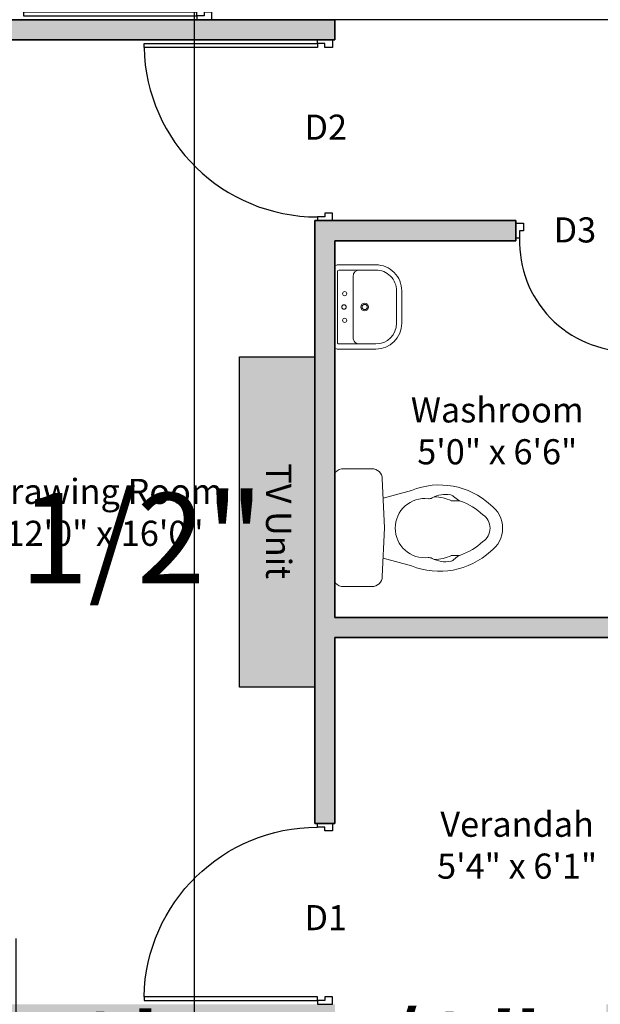
# Model space of a CAD drawing. Units: inches. Extents: x 2796 to 3603, y 978 to 1787.
# Tile 5 of 15: x 3165 to 3280, y 1116 to 1312. Entities that reach past the tile are written whole.
import ezdxf

# ---------------------------------------------------------------- set-up
doc = ezdxf.new("R2010")
doc.units = ezdxf.units.IN
for name, color, linetype, lineweight in [('A-ANNO-DIMS', 7, 'Continuous', 18), ('A-ANNO-TEXT', 7, 'Continuous', 18), ('A-AREA-IDEN', 7, 'Continuous', 18), ('A-DOOR', 6, 'Continuous', 25), ('A-FLOR-CASE', 2, 'Continuous', 25), ('A-FLOR-CASE-PATT', 2, 'Continuous', 13), ('A-FLOR-FIXT', 8, 'Continuous', 18), ('A-WALL-EXTR-PATT', 1, 'Continuous', 13), ('A-WALL-INTR-PATT', 5, 'Continuous', 13), ('Inner Wall', 5, 'Continuous', 35)]:
    doc.layers.add(name, color=color, linetype=linetype, lineweight=lineweight)
doc.styles.get("Standard").update_dxf_attribs({"font": 'arial.ttf'})
doc.dimstyles.get("Standard").update_dxf_attribs({"dimtxt": 18, "dimasz": 12, "dimexe": 0.18, "dimexo": 0.0625, "dimgap": 0.09, "dimtad": 0, "dimtih": 1, "dimtoh": 1, "dimdec": 0, "dimzin": 0, "dimdsep": 46, "dimlunit": 3, "dimtxsty": 'Standard', "dimcen": 0.09, "dimadec": 0, "dimazin": 0, "dimtfac": 1, "dimtdec": 0, "dimtofl": 0, "dimtmove": 0, "dimatfit": 3, "dimfxl": 1, "dimtolj": 1, "dimtzin": 0, "dimarcsym": 0})

# ---------------------------------------------------------------- blocks, each defined once
blk = doc.blocks.new('A$C57EA129C')
for p, q in [((0, 0.4428), (0, 0.1782)), ((0.016, 0.4589), (0.5631, 0.4589)), ((0.0356, 0.4321), (0.0356, 0.2896)), ((0.0445, 0.441), (0.5346, 0.441)), ((0.5435, 0.4321), (0.5435, 0.2896)), ((0.5791, 0.4428), (0.5791, 0.1782)), ((0.0356, 0.2896), (0.0356, 0.1782)), ((0.0802, 0.3341), (0.499, 0.3341)), ((0.5435, 0.2896), (0.5435, 0.1782)), ((0.1782, 0.0356), (0.4009, 0.0356)), ((0.1782, 0), (0.4009, 0))]:
    blk.add_line(p, q)
for centre, radius in [((0.1982, 0.392), 0.0143), ((0.2896, 0.3965), 0.0156), ((0.3809, 0.392), 0.0143), ((0.2896, 0.2545), 0.0267), ((0.2896, 0.2545), 0.0178)]:
    blk.add_circle(centre, radius)
for centre, radius, start, end in [((0.016, 0.4428), 0.016, 90, 180), ((0.0445, 0.4321), 0.00891, 90, 180), ((0.5346, 0.4321), 0.00891, 0, 90), ((0.5631, 0.4428), 0.016, 0, 90), ((0.0802, 0.2896), 0.0445, 90, 180), ((0.499, 0.2896), 0.0445, 0, 90), ((0.1782, 0.1782), 0.1782, 180, 270), ((0.1782, 0.1782), 0.1426, 180, 270), ((0.4009, 0.1782), 0.1782, 270, 0), ((0.4009, 0.1782), 0.1426, 270, 0)]:
    blk.add_arc(centre, radius, start, end)
blk = doc.blocks.new('A$C1308471B')
at = {"ltscale": 20}
for p, q in [((0, 0.4607), (0, 0.0186)), ((0.0354, 0.4793), (0.1495, 0.4793)), ((0.2013, 0.2397), (0.1923, 0.4384)), ((0.1957, 0.3639), (0.3109, 0.3953)), ((0.4982, 0.3575), (0.4822, 0.3709)), ((0.5021, 0.3528), (0.4724, 0.3528)), ((0.2013, 0.2397), (0.1923, 0.0409)), ((0.5021, 0.1304), (0.4724, 0.1304)), ((0.4982, 0.1257), (0.4822, 0.1123)), ((0.1959, 0.1193), (0.3109, 0.0879)), ((0.0354, 0), (0.1495, 0))]:
    blk.add_line(p, q, dxfattribs=at)
for centre, radius, start, end in [((0.006, 0.4607), 0.006, 136.5269, 180), ((0.0354, 0.4328), 0.0465, 90, 136.5269), ((0.1495, 0.4365), 0.0429, 2.5755, 90), ((0.4248, 0.1104), 0.3068, 47.4135, 111.7924), ((0.3654, 0.2416), 0.1206, 83.3523, 180), ((0.3823, 0.3868), 0.0255, 263.3523, 298.5742), ((0.4494, 0.2636), 0.1148, 79.3968, 118.5742), ((0.405, 0.2159), 0.153, 63.502, 90.4522), ((0.4658, 0.3513), 0.0255, 50, 79.3968), ((0.5146, 0.377), 0.0255, 230, 251.3881), ((0.5021, 0.3273), 0.0255, 70.3751, 90), ((0.4248, 0.1104), 0.2558, 46.612, 70.3751), ((0.5654, 0.2416), 0.116, 0, 54.7115), ((0.5654, 0.2416), 0.065, 0, 57.2974), ((0.3654, 0.2416), 0.1206, 180, 276.6477), ((0.5654, 0.2416), 0.065, 302.7026, 0), ((0.5654, 0.2416), 0.116, 305.2885, 0), ((0.4248, 0.3728), 0.2558, 289.6249, 313.388), ((0.4248, 0.3728), 0.3068, 248.2076, 312.5865), ((0.3823, 0.0964), 0.0255, 61.4258, 96.6477), ((0.405, 0.2673), 0.153, 269.5478, 296.498), ((0.5146, 0.1062), 0.0255, 108.6119, 130), ((0.5021, 0.1559), 0.0255, 270, 289.6249), ((0.4494, 0.2196), 0.1148, 241.4258, 280.6032), ((0.4658, 0.1319), 0.0255, 280.6032, 310), ((0.1495, 0.0429), 0.0429, 270, 357.4245), ((0.006, 0.0186), 0.006, 180, 223.4731), ((0.0354, 0.0465), 0.0465, 223.4731, 270)]:
    blk.add_arc(centre, radius, start, end, dxfattribs=at)
blk = doc.blocks.new('DOOR-SWING-36IN')
for points in [[(-0.01, 34.5), (-0.01, 0), (-0.76, 0), (-0.76, 34.5)], [(-35.26, -3), (-33.76, -3), (-33.76, -1.5), (-34.51, -1.5), (-34.51, 0), (-35.26, 0)], [(0.74, -3), (-0.76, -3), (-0.76, -1.5), (-0.01, -1.5), (-0.01, 0), (0.74, 0)]]:
    blk.add_lwpolyline(points, close=True)
blk.add_arc((0, 0), 34.51, 91.2592, 180)
blk = doc.blocks.new('DOOR-SWING-24IN')
for points in [[(-0.75, -0.7375), (-0.75, 21.7625), (0, 21.7625), (0, -0.7375)], [(-1.5, -3.7375), (0, -3.7375), (0, -2.2375), (-0.75, -2.2375), (-0.75, -0.7375), (-1.5, -0.7375)], [(22.5, -3.7375), (21, -3.7375), (21, -2.2375), (21.75, -2.2375), (21.75, -0.7375), (22.5, -0.7375)]]:
    blk.add_lwpolyline(points, close=True)
blk.add_arc((0, 0), 21.7625, 358.057956, 90)
blk = doc.blocks.new('TV-UNIT-66IN-NOM')
blk.add_lwpolyline([(0, 0), (65.77, 0), (65.77, -15), (0, -15)], close=True)
blk = doc.blocks.new('*D30')
at = {"layer": 'A-ANNO-DIMS', "color": 0, "lineweight": -2, "transparency": 16777216}
for p, q in [((3083.98, 1288.1), (3059.97, 1288.1)), ((3060.15, 1276.1), (3060.15, 1217.86)), ((3060.15, 1140.81), (3060.15, 1199.05)), ((3083.98, 1128.81), (3059.97, 1128.81))]:
    blk.add_line(p, q, dxfattribs=at)
at = {"layer": 'A-ANNO-DIMS', "color": 0, "transparency": 16777216}
for points in [[(3058.15, 1276.1), (3062.15, 1276.1), (3060.15, 1288.1)], [(3058.15, 1140.81), (3062.15, 1140.81), (3060.15, 1128.81)]]:
    blk.add_solid(points, dxfattribs=at)
at = {"layer": 'Defpoints', "color": 0, "transparency": 16777216}
for p in [(3084.05, 1288.1), (3060.15, 1128.81), (3084.05, 1128.81)]:
    blk.add_point(p, dxfattribs=at)
at = {"layer": 'A-ANNO-DIMS', "color": 0, "transparency": 16777216, "insert": (3060.15, 1208.46), "char_height": 18, "attachment_point": 5}
blk.add_mtext('\\A1;SEATING GROUP 13\'-3 1/2"', dxfattribs=at)
blk = doc.blocks.new('*D31')
at = {"layer": 'A-ANNO-DIMS', "color": 0, "lineweight": -2, "transparency": 16777216}
for p, q in [((3084.05, 1128.75), (3084.05, 1104.74)), ((3163.77, 1128.75), (3163.77, 1104.74)), ((3096.05, 1104.92), (3151.77, 1104.92)), ((3163.77, 1104.92), (3175.77, 1104.92))]:
    blk.add_line(p, q, dxfattribs=at)
at = {"layer": 'A-ANNO-DIMS', "color": 0, "transparency": 16777216}
for points in [[(3096.05, 1106.92), (3096.05, 1102.92), (3084.05, 1104.92)], [(3151.77, 1106.92), (3151.77, 1102.92), (3163.77, 1104.92)]]:
    blk.add_solid(points, dxfattribs=at)
at = {"layer": 'Defpoints', "color": 0, "transparency": 16777216}
for p in [(3084.05, 1128.81), (3163.77, 1128.81), (3163.77, 1104.92)]:
    blk.add_point(p, dxfattribs=at)
at = {"layer": 'A-ANNO-DIMS', "color": 0, "transparency": 16777216, "insert": (3220.81, 1104.92), "char_height": 18, "attachment_point": 5}
blk.add_mtext('\\A1;6\'-7 1/2"', dxfattribs=at)
blk = doc.blocks.new('*D34')
at = {"layer": 'A-ANNO-DIMS', "color": 0, "lineweight": -2, "transparency": 16777216}
for p, q in [((3355.83, 1336.87), (3343.83, 1336.87)), ((3355.83, 1332.81), (3355.83, 1337.05)), ((3371.32, 1336.87), (3367.83, 1336.87)), ((3383.32, 1332.81), (3383.32, 1337.05))]:
    blk.add_line(p, q, dxfattribs=at)
at = {"layer": 'A-ANNO-DIMS', "color": 0, "transparency": 16777216}
for points in [[(3367.83, 1338.87), (3367.83, 1334.87), (3355.83, 1336.87)], [(3371.32, 1338.87), (3371.32, 1334.87), (3383.32, 1336.87)]]:
    blk.add_solid(points, dxfattribs=at)
at = {"layer": 'Defpoints', "color": 0, "transparency": 16777216}
for p in [(3355.83, 1336.87), (3355.83, 1332.75), (3383.32, 1332.75)]:
    blk.add_point(p, dxfattribs=at)
at = {"layer": 'A-ANNO-DIMS', "color": 0, "transparency": 16777216, "insert": (3268.59, 1336.87), "char_height": 18, "attachment_point": 5}
blk.add_mtext('\\A1;HOB 2\'-3 1/2"', dxfattribs=at)
blk = doc.blocks.new('*D51')
at = {"layer": 'A-ANNO-DIMS', "color": 0, "lineweight": -2, "transparency": 16777216}
for p, q in [((3127.245499, 1431.61284), (3127.245499, 989.79534)), ((3199.245499, 1431.61284), (3199.245499, 989.79534)), ((3115.245499, 989.97534), (3103.245499, 989.97534)), ((3211.245499, 989.97534), (3223.245499, 989.97534))]:
    blk.add_line(p, q, dxfattribs=at)
at = {"layer": 'A-ANNO-DIMS', "color": 0, "transparency": 16777216}
for points in [[(3115.245499, 991.97534), (3115.245499, 987.97534), (3127.245499, 989.97534)], [(3211.245499, 991.97534), (3211.245499, 987.97534), (3199.245499, 989.97534)]]:
    blk.add_solid(points, dxfattribs=at)
at = {"layer": 'Defpoints', "color": 0, "transparency": 16777216}
for p in [(3127.245499, 1431.67534), (3199.245499, 1431.67534), (3199.245499, 989.97534)]:
    blk.add_point(p, dxfattribs=at)
at = {"layer": 'A-ANNO-DIMS', "color": 0, "transparency": 16777216, "insert": (3163.245499, 989.97534), "char_height": 18, "attachment_point": 5}
blk.add_mtext('\\A1;6\'-0"', dxfattribs=at)
blk = doc.blocks.new('*D53')
at = {"layer": 'A-ANNO-DIMS', "color": 0, "lineweight": -2, "transparency": 16777216}
for p, q in [((3031.545499, 1347.67534), (3031.545499, 1359.67534)), ((3333.182999, 1335.67534), (3031.365499, 1335.67534)), ((3333.182999, 1311.67534), (3031.365499, 1311.67534)), ((3031.545499, 1299.67534), (3031.545499, 1287.67534))]:
    blk.add_line(p, q, dxfattribs=at)
at = {"layer": 'A-ANNO-DIMS', "color": 0, "transparency": 16777216}
for points in [[(3029.545499, 1347.67534), (3033.545499, 1347.67534), (3031.545499, 1335.67534)], [(3029.545499, 1299.67534), (3033.545499, 1299.67534), (3031.545499, 1311.67534)]]:
    blk.add_solid(points, dxfattribs=at)
at = {"layer": 'Defpoints', "color": 0, "transparency": 16777216}
for p in [(3031.545499, 1335.67534), (3333.245499, 1335.67534), (3333.245499, 1311.67534)]:
    blk.add_point(p, dxfattribs=at)
at = {"layer": 'A-ANNO-DIMS', "color": 0, "transparency": 16777216, "insert": (3031.545499, 1323.67534), "char_height": 18, "attachment_point": 5}
blk.add_mtext('\\A1;2\'-0"', dxfattribs=at)

msp = doc.modelspace()

# ---------------------------------------------------------------- hatches: boundary and pattern name
at = {"layer": 'A-FLOR-CASE-PATT'}
h = msp.add_hatch(dxfattribs=at)
h.set_pattern_fill('GOST_WOOD', color=256)
h.paths.add_polyline_path([(3127.25, 1727.68), (3079.25, 1727.68), (3079.25, 1703.68), (3127.25, 1703.68)])
h.paths.add_polyline_path([(3245.25, 1629.3), (3230.25, 1629.3), (3230.25, 1563.53), (3245.25, 1563.53)])
h.paths.add_polyline_path([(3381.25, 1651.68), (3315.48, 1651.68), (3315.48, 1636.68), (3381.25, 1636.68)])
h.paths.add_polyline_path([(3415.25, 1603.68), (3391.25, 1603.68), (3391.25, 1507.68), (3415.25, 1507.68)])
h.paths.add_polyline_path([(3199.25, 1407.44), (3184.25, 1407.44), (3184.25, 1353.68), (3199.25, 1353.68)])
h.paths.add_polyline_path([(3199.25, 1455.68), (3127.25, 1455.68), (3127.25, 1431.68), (3199.25, 1431.68)])
h.paths.add_polyline_path([(3223.25, 1244.56), (3208.25, 1244.56), (3208.25, 1178.79), (3223.25, 1178.79)])
h.paths.add_polyline_path([(3093.36, 1710.13), (3112.68, 1710.13), (3112.68, 1720.81), (3093.36, 1720.81)], flags=24)
h.paths.add_polyline_path([(3232.57, 1610.37), (3232.57, 1583.04), (3243.25, 1583.04), (3243.25, 1610.37)], flags=24)
h.paths.add_polyline_path([(3334.41, 1639), (3361.73, 1639), (3361.73, 1649.68), (3334.41, 1649.68)], flags=24)
h.paths.add_polyline_path([(3398.2, 1565.36), (3398.2, 1546.04), (3408.87, 1546.04), (3408.87, 1565.36)], flags=24)
h.paths.add_polyline_path([(3186.57, 1394.51), (3186.57, 1367.19), (3197.25, 1367.19), (3197.25, 1394.51)], flags=24)
h.paths.add_polyline_path([(3153.56, 1438.63), (3172.88, 1438.63), (3172.88, 1449.3), (3153.56, 1449.3)], flags=24)
h.paths.add_polyline_path([(3210.57, 1225.63), (3210.57, 1198.3), (3221.25, 1198.3), (3221.25, 1225.63)], flags=24)
at = {"layer": 'A-WALL-EXTR-PATT'}
h = msp.add_hatch(color=256, dxfattribs=at)
h.dxf.hatch_style = 1
h.paths.add_polyline_path([(3424.25, 1736.68), (3070.25, 1736.68), (3070.25, 1106.68), (3227.25, 1106.68), (3227.25, 1115.68), (3226.75, 1115.68), (3223.75, 1115.68), (3079.25, 1115.68), (3079.25, 1727.68), (3127.25, 1727.68), (3415.25, 1727.68), (3415.25, 1188.68), (3424.25, 1188.68)])
h.paths.add_polyline_path([(3291.25, 1032.68), (3074.25, 1032.68), (3074.25, 1106.68), (3070.25, 1106.68), (3070.25, 1028.68), (3291.25, 1028.68)])
h.paths.add_polyline_path([(3291.25, 1115.68), (3281.25, 1115.68), (3281.25, 1106.68), (3291.25, 1106.68)], flags=17)
h.paths.add_polyline_path([(3301.25, 1037.68), (3291.25, 1037.68), (3291.25, 1028.68), (3301.25, 1028.68)])
h.paths.add_polyline_path([(3424.25, 1037.68), (3414.25, 1037.68), (3414.25, 1028.68), (3424.25, 1028.68)])
h.paths.add_polyline_path([(3424.25, 1188.68), (3420.25, 1188.68), (3420.25, 1037.68), (3424.25, 1037.68)])
at = {"layer": 'A-WALL-INTR-PATT'}
h = msp.add_hatch(color=256, dxfattribs=at)
h.dxf.hatch_style = 1
h.paths.add_polyline_path([(3249.25, 1727.68), (3245.25, 1727.68), (3245.25, 1655.68), (3103.25, 1655.68), (3103.25, 1651.68), (3245.25, 1651.68), (3245.25, 1503.68), (3249.25, 1503.68)])
h.paths.add_polyline_path([(3131.25, 1727.68), (3127.25, 1727.68), (3127.25, 1703.68), (3127.25, 1679.68), (3131.25, 1679.68)], flags=17)
h.paths.add_polyline_path([(3391.25, 1655.68), (3325.25, 1655.68), (3325.25, 1727.68), (3321.25, 1727.68), (3321.25, 1655.68), (3273.25, 1655.68), (3273.25, 1651.68), (3391.25, 1651.68)])
h.paths.add_polyline_path([(3203.25, 1459.68), (3079.25, 1459.68), (3079.25, 1455.68), (3199.25, 1455.68), (3199.25, 1431.68), (3199.25, 1347.68), (3203.25, 1347.68)])
h.paths.add_polyline_path([(3209.25, 1507.68), (3079.25, 1507.68), (3079.25, 1503.68), (3209.25, 1503.68)])
h.paths.add_polyline_path([(3415.25, 1507.68), (3285.25, 1507.68), (3285.25, 1503.68), (3415.25, 1503.68)])
h.paths.add_polyline_path([(3415.25, 1459.68), (3333.25, 1459.68), (3333.25, 1455.68), (3415.25, 1455.68)])
h.paths.add_polyline_path([(3291.25, 1311.68), (3287.25, 1311.68), (3287.25, 1192.68), (3227.25, 1192.68), (3227.25, 1267.68), (3263.25, 1267.68), (3263.25, 1271.68), (3223.25, 1271.68), (3223.25, 1151.68), (3227.25, 1151.68), (3227.25, 1188.68), (3291.25, 1188.68)])
h.paths.add_polyline_path([(3227.25, 1311.68), (3079.25, 1311.68), (3079.25, 1307.68), (3227.25, 1307.68)])

# ---------------------------------------------------------------- linework, layer by layer
at = {"layer": 'Inner Wall'}
for p, q in [((3079.25, 1311.68), (3227.25, 1311.68)), ((3227.25, 1307.68), (3227.25, 1311.68)), ((3079.25, 1307.68), (3227.25, 1307.68)), ((3223.25, 1151.68), (3223.25, 1271.68)), ((3223.25, 1271.68), (3263.25, 1271.68)), ((3263.25, 1267.68), (3263.25, 1271.68)), ((3227.25, 1192.68), (3227.25, 1267.68)), ((3227.25, 1267.68), (3263.25, 1267.68)), ((3227.25, 1192.68), (3287.25, 1192.68)), ((3227.25, 1188.68), (3291.25, 1188.68)), ((3227.25, 1151.68), (3227.25, 1188.68)), ((3223.25, 1151.68), (3227.25, 1151.68))]:
    msp.add_line(p, q, dxfattribs=at)

# ---------------------------------------------------------------- block references
at = {"layer": 'A-DOOR', "extrusion": (0, 0, -1), "zscale": -1}
for p, rotation in [((-3199.75, 1312.42), 269.9999999999978), ((-3223.75, 1116.42), 269.9999999999984)]:
    msp.add_blockref('DOOR-SWING-36IN', p, dxfattribs=dict(at, rotation=rotation))
at = {"layer": 'A-DOOR'}
for name, p, rotation in [('DOOR-SWING-36IN', (3223.75, 1306.93), 89.99999999999916), ('DOOR-SWING-24IN', (3285.75, 1267.44), 180)]:
    msp.add_blockref(name, p, dxfattribs=dict(at, rotation=rotation))
at = {"layer": 'A-FLOR-CASE', "rotation": 269.9999999999993}
msp.add_blockref('TV-UNIT-66IN-NOM', (3223.25, 1244.56), dxfattribs=at)
at = {"layer": 'A-FLOR-FIXT'}
for name, p, xscale, yscale, zscale, rotation in [('A$C57EA129C', (3240.54, 1246.09), 28.98333223671166, 28.98333223671166, 28.98333223671166, 89.99999999999999), ('A$C1308471B', (3227.25, 1222.29), -48.95497407897215, 48.95497407897215, 48.95497407897215, 180)]:
    msp.add_blockref(name, p, dxfattribs=dict(at, xscale=xscale, yscale=yscale, zscale=zscale, rotation=rotation))

# ---------------------------------------------------------------- texts
at = {"layer": 'A-ANNO-TEXT', "char_height": 5, "attachment_point": 3}
for s, insert in [('\\pxqc;{\\fTimes New Roman|b0|i0|c0|p18;D2}', (3233.25, 1292.78)), ('\\pxqc;{\\fTimes New Roman|b0|i0|c0|p18;D3}', (3282.83, 1272.33)), ('\\pxqc;{\\fTimes New Roman|b0|i0|c0|p18;D1}', (3233.25, 1135.43))]:
    msp.add_mtext_dynamic_manual_height_columns(s, width=15.6741, gutter_width=12.5, heights=[0], dxfattribs=dict(at, insert=insert))
at = {"layer": 'A-ANNO-TEXT', "insert": (3218.54, 1194.24), "char_height": 5, "attachment_point": 3, "rotation": 270}
msp.add_mtext_dynamic_manual_height_columns('\\pxqc;{\\fTimes New Roman|b0|i0|c0|p18;TV Unit}', width=35.2337, gutter_width=12.5, heights=[0], dxfattribs=at)
at = {"layer": 'A-AREA-IDEN', "char_height": 5, "attachment_point": 3}
for s, width, insert in [('\\pxqc;{\\fTimes New Roman|b0|i0|c0|p18;Washroom\\P5\'0" x 6\'6"}', 35.2337, (3277.16, 1236.5)), ('\\pxqc;{\\fTimes New Roman|b0|i0|c0|p18;Drawing Room\\P12\'0" x 16\'0"}', 55.5021, (3209.15, 1220.27)), ('\\pxqc;{\\fTimes New Roman|b0|i0|c0|p18;Verandah\\P5\'4" x 6\'1"}', 55.5021, (3291.25, 1154.02))]:
    msp.add_mtext_dynamic_manual_height_columns(s, width=width, gutter_width=12.5, heights=[0], dxfattribs=dict(at, insert=insert))

# ---------------------------------------------------------------- dimensions: what is measured, and where the dimension line sits
at = {"layer": 'A-ANNO-DIMS'}
for base, p1, p2, picture, middle in [((3199.25, 989.98), (3127.25, 1431.68), (3199.25, 1431.68), '*D51', (3163.25, 989.98)), ((3163.77, 1104.92), (3084.05, 1128.81), (3163.77, 1128.81), '*D31', (3220.81, 1104.92))]:
    dim = msp.add_linear_dim(base=base, p1=p1, p2=p2, dimstyle='Standard', override={"dimdec": 1, "dimlfac": 1, "dimrnd": 0, "dimzin": 1, "dimdsep": 46, "dimlunit": 4, "dimfrac": 2}, dxfattribs=at)
    dim.commit()
    dim.dimension.update_dxf_attribs({"geometry": picture, "text_midpoint": middle})
for base, p1, p2, angle, text, picture, middle in [((3355.83, 1336.87), (3383.32, 1332.75), (3355.83, 1332.75), 180, 'HOB <>', '*D34', (3268.59, 1336.87)), ((3060.15, 1128.81), (3084.05, 1288.1), (3084.05, 1128.81), 270, 'SEATING GROUP <>', '*D30', (3060.15, 1208.46))]:
    dim = msp.add_linear_dim(base=base, p1=p1, p2=p2, angle=angle, text=text, dimstyle='Standard', override={"dimdec": 1, "dimlfac": 1, "dimrnd": 0, "dimzin": 1, "dimdsep": 46, "dimlunit": 4, "dimfrac": 2}, dxfattribs=at)
    dim.commit()
    dim.dimension.update_dxf_attribs({"geometry": picture, "text_midpoint": middle})
dim = msp.add_linear_dim(base=(3031.55, 1335.68), p1=(3333.25, 1311.68), p2=(3333.25, 1335.68), angle=90, dimstyle='Standard', override={"dimdec": 1, "dimlfac": 1, "dimrnd": 0, "dimzin": 1, "dimdsep": 46, "dimlunit": 4, "dimfrac": 2}, dxfattribs=at)
dim.commit()
dim.dimension.update_dxf_attribs({"geometry": '*D53', "text_midpoint": (3031.55, 1323.68)})

doc.saveas('drawing.dxf')
